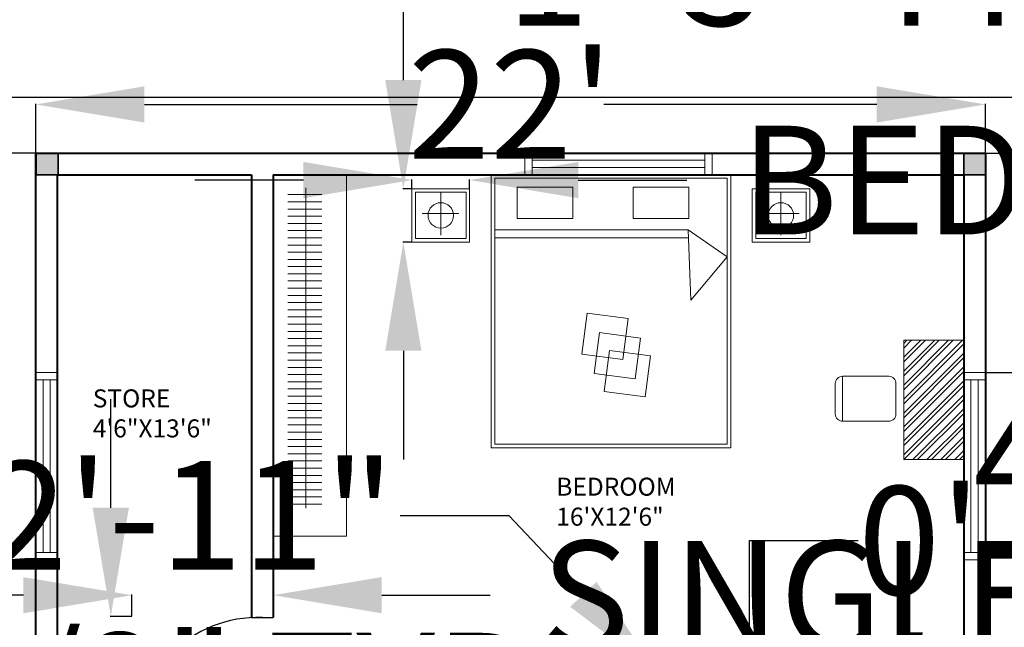
# Model space of a CAD drawing. Units: inches. Extents: x 7323 to 9737, y 2037 to 3322.
# Tile 6 of 19: x 8647 to 8921, y 2540 to 2709. Entities that reach past the tile are written whole.
import ezdxf

# ---------------------------------------------------------------- set-up
doc = ezdxf.new("R2010")
doc.units = ezdxf.units.IN
doc.header["$MEASUREMENT"] = 0
for name, color, linetype, lineweight in [('A-ANNO-DIMS', 2, 'Continuous', 18), ('A-AREA-IDEN', 7, 'Continuous', 18), ('A-COLS', 1, 'Continuous', 35), ('A-DOOR', 4, 'Continuous', 25), ('A-FLOR-CASE', 9, 'Continuous', 20), ('A-FLOR-CASE-PATT', 8, 'Continuous', 13), ('A-FURN', 8, 'Continuous', 18), ('A-FURN-PATT', 252, 'Continuous', 13), ('A-GLAZ', 4, 'Continuous', 18), ('A-WALL', 7, 'Continuous', 40)]:
    doc.layers.add(name, color=color, linetype=linetype, lineweight=lineweight)
doc.layers.add('A-COLS-PATT', color=18, linetype='Continuous', lineweight=13, true_color=0x000000)
doc.styles.get("Standard").update_dxf_attribs({"font": 'arial.ttf'})
doc.dimstyles.get("Standard").update_dxf_attribs({"dimtxt": 30.18, "dimasz": 30.18, "dimexe": 0.18, "dimexo": 0.0625, "dimgap": 0.09, "dimtad": 0, "dimtih": 1, "dimtoh": 1, "dimdec": 0, "dimzin": 0, "dimdsep": 46, "dimlunit": 3, "dimtxsty": 'Standard', "dimcen": 0.09, "dimadec": 0, "dimazin": 0, "dimtfac": 1, "dimtdec": 0, "dimtofl": 0, "dimtmove": 0, "dimatfit": 3, "dimfxl": 1, "dimtolj": 1, "dimtzin": 0, "dimarcsym": 0})

# ---------------------------------------------------------------- blocks, each defined once
blk = doc.blocks.new('*D9')
at = {"layer": 'A-ANNO-DIMS', "color": 0, "lineweight": -2, "transparency": 16777216}
for p, q in [((8651.39, 2671.93), (8651.39, 2685.56)), ((8915.39, 2671.93), (8915.39, 2685.56)), ((8681.57, 2685.38), (8757.44, 2685.38)), ((8885.21, 2685.38), (8809.35, 2685.38))]:
    blk.add_line(p, q, dxfattribs=at)
at = {"layer": 'A-ANNO-DIMS', "color": 0, "transparency": 16777216}
for points in [[(8681.57, 2690.41), (8681.57, 2680.35), (8651.39, 2685.38)], [(8885.21, 2690.41), (8885.21, 2680.35), (8915.39, 2685.38)]]:
    blk.add_solid(points, dxfattribs=at)
at = {"layer": 'Defpoints', "color": 0, "transparency": 16777216}
for p in [(8915.39, 2685.38), (8651.39, 2671.86), (8915.39, 2671.86)]:
    blk.add_point(p, dxfattribs=at)
at = {"layer": 'A-ANNO-DIMS', "color": 0, "transparency": 16777216, "insert": (8783.39, 2685.38), "char_height": 30.18, "attachment_point": 5}
blk.add_mtext("\\A1;22'", dxfattribs=at)
blk = doc.blocks.new('WIN-48')
for p, q in [((0, 0), (0, 6)), ((2, 0), (2, 6)), ((50, 0), (50, 6)), ((52, 0), (52, 6)), ((2, 4), (50, 4)), ((2, 2), (50, 2))]:
    blk.add_line(p, q)
blk = doc.blocks.new('DOOR-36')
for p, q in [((33.01, 39), (39.01, 39)), ((36.01, 5), (0.01, 5)), ((33.01, 3), (0.01, 3)), ((36.01, 5), (36.01, 3)), ((36.01, 3), (39.01, 3)), ((33.01, 0), (39.01, 0))]:
    blk.add_line(p, q)
blk.add_arc((35.01, 4), 35.01, 88.3634, 181.6366)
blk = doc.blocks.new('BED-DOUBLE-REAR')
for p, q in [((1, 60.58), (54.75, 60.58)), ((54.75, 60.58), (65.65, 53.04)), ((55.5, 41.06), (54.75, 60.58)), ((54.83, 58.32), (1, 58.32)), ((65.65, 53.04), (55.5, 41.06))]:
    blk.add_line(p, q)
for points in [[(0, 75.91), (66.65, 75.91), (66.65, 0), (0, 0)], [(1, 74.91), (65.65, 74.91), (65.65, 1), (1, 1)], [(7.24, 72.42), (22.67, 72.42), (22.67, 63.7), (7.24, 63.7)], [(39.52, 72.42), (54.95, 72.42), (54.95, 63.7), (39.52, 63.7)], [(36.59, 24.55), (38.1, 35.92), (26.73, 37.42), (25.22, 26.05)], [(40.02, 19.16), (41.52, 30.53), (30.15, 32.04), (28.64, 20.66)], [(42.82, 14.19), (44.32, 25.56), (32.95, 27.06), (31.44, 15.69)]]:
    blk.add_lwpolyline(points, close=True)
blk = doc.blocks.new('BEDSIDE-TABLE-LARGE')
for p, q in [((8.01, 13.84), (8.01, 1.98)), ((2.84, 7.91), (13.05, 7.91))]:
    blk.add_line(p, q)
for points in [[(0, 14.84), (16.03, 14.84), (16.03, 0), (0, 0)], [(1, 13.84), (15.03, 13.84), (15.03, 1), (1, 1)]]:
    blk.add_lwpolyline(points, close=True)
blk.add_circle((8.01, 7.42), 3.54)
blk = doc.blocks.new('COL-PLAN-6IN')
blk.add_lwpolyline([(0, 6), (0, 6), (6.06, 6), (6.06, 6), (6.06, 0), (6.06, 0), (0, 0), (0, 0)], close=True)
blk = doc.blocks.new('*D39')
at = {"layer": 'A-ANNO-DIMS', "color": 0, "lineweight": -2, "transparency": 16777216}
for p, q in [((8647.94, 2549.03), (8617.76, 2549.03)), ((8678.12, 2543.2), (8678.12, 2549.21)), ((8717.39, 2543.2), (8717.39, 2549.21)), ((8747.57, 2549.03), (8777.75, 2549.03))]:
    blk.add_line(p, q, dxfattribs=at)
at = {"layer": 'A-ANNO-DIMS', "color": 0, "transparency": 16777216}
for points in [[(8647.94, 2554.06), (8647.94, 2544), (8678.12, 2549.03)], [(8747.57, 2554.06), (8747.57, 2544), (8717.39, 2549.03)]]:
    blk.add_solid(points, dxfattribs=at)
at = {"layer": 'Defpoints', "color": 0, "transparency": 16777216}
for p in [(8717.39, 2549.03), (8678.12, 2543.14), (8717.39, 2543.14)]:
    blk.add_point(p, dxfattribs=at)
at = {"layer": 'A-ANNO-DIMS', "color": 0, "transparency": 16777216, "insert": (9057.19, 2549.03), "char_height": 30.18, "attachment_point": 5}
blk.add_mtext('\\A1;SINGLE DOOR 3\'-3 1/2" TYP.', dxfattribs=at)
blk = doc.blocks.new('*D40')
at = {"layer": 'A-ANNO-DIMS', "color": 0, "lineweight": -2, "transparency": 16777216}
for p, q in [((8672.23, 2573.32), (8672.23, 2603.5)), ((8678.06, 2543.14), (8672.05, 2543.14)), ((8678.06, 2503.86), (8672.05, 2503.86)), ((8672.23, 2473.68), (8672.23, 2443.5))]:
    blk.add_line(p, q, dxfattribs=at)
at = {"layer": 'A-ANNO-DIMS', "color": 0, "transparency": 16777216}
for points in [[(8667.2, 2573.32), (8677.26, 2573.32), (8672.23, 2543.14)], [(8667.2, 2473.68), (8677.26, 2473.68), (8672.23, 2503.86)]]:
    blk.add_solid(points, dxfattribs=at)
at = {"layer": 'Defpoints', "color": 0, "transparency": 16777216}
for p in [(8672.23, 2543.14), (8678.12, 2543.14), (8678.12, 2503.86)]:
    blk.add_point(p, dxfattribs=at)
at = {"layer": 'A-ANNO-DIMS', "color": 0, "transparency": 16777216, "insert": (8672.23, 2523.5), "char_height": 30.18, "attachment_point": 5}
blk.add_mtext('\\A1;3\'-3 1/2" TYP.', dxfattribs=at)
blk = doc.blocks.new('*D41')
at = {"layer": 'A-ANNO-DIMS', "color": 0, "lineweight": -2, "transparency": 16777216}
for p, q in [((8661.59, 2428.04), (8661.59, 2458.22)), ((8661.59, 2458.22), (8691.77, 2458.22)), ((8657.46, 2397.86), (8661.77, 2397.86)), ((8657.46, 2369.86), (8661.77, 2369.86)), ((8661.59, 2339.68), (8661.59, 2309.5))]:
    blk.add_line(p, q, dxfattribs=at)
at = {"layer": 'A-ANNO-DIMS', "color": 0, "transparency": 16777216}
for points in [[(8656.56, 2428.04), (8666.62, 2428.04), (8661.59, 2397.86)], [(8656.56, 2339.68), (8666.62, 2339.68), (8661.59, 2369.86)]]:
    blk.add_solid(points, dxfattribs=at)
at = {"layer": 'Defpoints', "color": 0, "transparency": 16777216}
for p in [(8657.39, 2397.86), (8661.59, 2397.86), (8657.39, 2369.86)]:
    blk.add_point(p, dxfattribs=at)
at = {"layer": 'A-ANNO-DIMS', "color": 0, "transparency": 16777216, "insert": (8945.06, 2458.22), "char_height": 30.18, "attachment_point": 5}
blk.add_mtext('\\A1;VENT WINDOW 2\'-4" TYP.', dxfattribs=at)
blk = doc.blocks.new('*D45')
at = {"layer": 'A-ANNO-DIMS', "color": 0, "lineweight": -2, "transparency": 16777216}
for p, q in [((8725.79, 2664.36), (8695.61, 2664.36)), ((8755.97, 2662.02), (8755.97, 2664.54)), ((8772, 2662.02), (8772, 2664.54)), ((8802.18, 2664.36), (8832.36, 2664.36))]:
    blk.add_line(p, q, dxfattribs=at)
at = {"layer": 'A-ANNO-DIMS', "color": 0, "transparency": 16777216}
for points in [[(8725.79, 2669.39), (8725.79, 2659.33), (8755.97, 2664.36)], [(8802.18, 2669.39), (8802.18, 2659.33), (8772, 2664.36)]]:
    blk.add_solid(points, dxfattribs=at)
at = {"layer": 'Defpoints', "color": 0, "transparency": 16777216}
for p in [(8772, 2664.36), (8755.97, 2661.96), (8772, 2661.96)]:
    blk.add_point(p, dxfattribs=at)
at = {"layer": 'A-ANNO-DIMS', "color": 0, "transparency": 16777216, "insert": (9094.8, 2664.36), "char_height": 30.18, "attachment_point": 5}
blk.add_mtext('\\A1;BEDSIDE TABLE 1\'-4" TYP.', dxfattribs=at)
blk = doc.blocks.new('*D46')
at = {"layer": 'A-ANNO-DIMS', "color": 0, "lineweight": -2, "transparency": 16777216}
for p, q in [((8753.57, 2692.14), (8753.57, 2722.32)), ((8753.57, 2722.32), (8783.75, 2722.32)), ((8755.91, 2661.96), (8753.39, 2661.96)), ((8755.91, 2647.12), (8753.39, 2647.12)), ((8753.57, 2616.94), (8753.57, 2586.76))]:
    blk.add_line(p, q, dxfattribs=at)
at = {"layer": 'A-ANNO-DIMS', "color": 0, "transparency": 16777216}
for points in [[(8748.54, 2692.14), (8758.6, 2692.14), (8753.57, 2661.96)], [(8748.54, 2616.94), (8758.6, 2616.94), (8753.57, 2647.12)]]:
    blk.add_solid(points, dxfattribs=at)
at = {"layer": 'Defpoints', "color": 0, "transparency": 16777216}
for p in [(8753.57, 2661.96), (8755.97, 2661.96), (8755.97, 2647.12)]:
    blk.add_point(p, dxfattribs=at)
at = {"layer": 'A-ANNO-DIMS', "color": 0, "transparency": 16777216, "insert": (8874.4, 2722.32), "char_height": 30.18, "attachment_point": 5}
blk.add_mtext('\\A1;1\'-3" TYP.', dxfattribs=at)
blk = doc.blocks.new('*D47')
at = {"layer": 'A-ANNO-DIMS', "color": 0, "lineweight": -2, "transparency": 16777216}
for p, q in [((8809.55, 2464.49), (8779.37, 2464.49)), ((8839.73, 2461.79), (8839.73, 2464.67)), ((8858.14, 2461.79), (8858.14, 2464.67)), ((8888.32, 2464.49), (8918.5, 2464.49))]:
    blk.add_line(p, q, dxfattribs=at)
at = {"layer": 'A-ANNO-DIMS', "color": 0, "transparency": 16777216}
for points in [[(8809.55, 2469.52), (8809.55, 2459.46), (8839.73, 2464.49)], [(8888.32, 2469.52), (8888.32, 2459.46), (8858.14, 2464.49)]]:
    blk.add_solid(points, dxfattribs=at)
at = {"layer": 'Defpoints', "color": 0, "transparency": 16777216}
for p in [(8858.14, 2464.49), (8839.73, 2461.73), (8858.14, 2461.73)]:
    blk.add_point(p, dxfattribs=at)
at = {"layer": 'A-ANNO-DIMS', "color": 0, "transparency": 16777216, "insert": (9164.9, 2464.49), "char_height": 30.18, "attachment_point": 5}
blk.add_mtext('\\A1;ARMCHAIR 1\'-6 1/2" TYP.', dxfattribs=at)
blk = doc.blocks.new('*D48')
at = {"layer": 'A-ANNO-DIMS', "color": 0, "lineweight": -2, "transparency": 16777216}
for p, q in [((8836.96, 2491.91), (8836.96, 2522.09)), ((8836.96, 2522.09), (8867.14, 2522.09)), ((8839.66, 2461.73), (8836.78, 2461.73)), ((8839.66, 2451.75), (8836.78, 2451.75)), ((8836.96, 2421.57), (8836.96, 2391.39))]:
    blk.add_line(p, q, dxfattribs=at)
at = {"layer": 'A-ANNO-DIMS', "color": 0, "transparency": 16777216}
for points in [[(8831.93, 2491.91), (8841.99, 2491.91), (8836.96, 2461.73)], [(8831.93, 2421.57), (8841.99, 2421.57), (8836.96, 2451.75)]]:
    blk.add_solid(points, dxfattribs=at)
at = {"layer": 'Defpoints', "color": 0, "transparency": 16777216}
for p in [(8836.96, 2461.73), (8839.73, 2461.73), (8839.73, 2451.75)]:
    blk.add_point(p, dxfattribs=at)
at = {"layer": 'A-ANNO-DIMS', "color": 0, "transparency": 16777216, "insert": (8970.94, 2522.09), "char_height": 30.18, "attachment_point": 5}
blk.add_mtext('\\A1;0\'-10" TYP.', dxfattribs=at)
blk = doc.blocks.new('*D53')
at = {"layer": 'A-ANNO-DIMS', "color": 0, "lineweight": -2, "transparency": 16777216}
for p, q in [((8826.85, 2511.06), (8796.67, 2511.06)), ((8857.03, 2503.93), (8857.03, 2511.24)), ((8905.03, 2503.93), (8905.03, 2511.24)), ((8935.21, 2511.06), (8965.39, 2511.06))]:
    blk.add_line(p, q, dxfattribs=at)
at = {"layer": 'A-ANNO-DIMS', "color": 0, "transparency": 16777216}
for points in [[(8826.85, 2516.09), (8826.85, 2506.03), (8857.03, 2511.06)], [(8935.21, 2516.09), (8935.21, 2506.03), (8905.03, 2511.06)]]:
    blk.add_solid(points, dxfattribs=at)
at = {"layer": 'Defpoints', "color": 0, "transparency": 16777216}
for p in [(8905.03, 2511.06), (8857.03, 2503.86), (8905.03, 2503.86)]:
    blk.add_point(p, dxfattribs=at)
at = {"layer": 'A-ANNO-DIMS', "color": 0, "transparency": 16777216, "insert": (9261.3, 2511.06), "char_height": 30.18, "attachment_point": 5}
blk.add_mtext('\\A1;INTERIOR WINDOW 4\'-0" TYP.', dxfattribs=at)
blk = doc.blocks.new('*D54')
at = {"layer": 'A-ANNO-DIMS', "color": 0, "lineweight": -2, "transparency": 16777216}
for p, q in [((8849.83, 2534.04), (8849.83, 2564.22)), ((8849.83, 2564.22), (8880.01, 2564.22)), ((8856.96, 2503.86), (8849.65, 2503.86)), ((8856.96, 2497.86), (8849.65, 2497.86)), ((8849.83, 2467.68), (8849.83, 2437.5))]:
    blk.add_line(p, q, dxfattribs=at)
at = {"layer": 'A-ANNO-DIMS', "color": 0, "transparency": 16777216}
for points in [[(8844.8, 2534.04), (8854.86, 2534.04), (8849.83, 2503.86)], [(8844.8, 2467.68), (8854.86, 2467.68), (8849.83, 2497.86)]]:
    blk.add_solid(points, dxfattribs=at)
at = {"layer": 'Defpoints', "color": 0, "transparency": 16777216}
for p in [(8849.83, 2503.86), (8857.03, 2503.86), (8857.03, 2497.86)]:
    blk.add_point(p, dxfattribs=at)
at = {"layer": 'A-ANNO-DIMS', "color": 0, "transparency": 16777216, "insert": (8972.08, 2564.22), "char_height": 30.18, "attachment_point": 5}
blk.add_mtext('\\A1;0\'-6" TYP.', dxfattribs=at)
blk = doc.blocks.new('*D63')
at = {"layer": 'A-ANNO-DIMS', "color": 0, "lineweight": -2, "transparency": 16777216}
for p, q in [((8744.72, 2466.22), (8744.72, 2496.4)), ((8744.72, 2496.4), (8774.9, 2496.4)), ((8741.46, 2436.04), (8744.9, 2436.04)), ((8741.46, 2413.86), (8744.9, 2413.86)), ((8744.72, 2383.68), (8744.72, 2353.5))]:
    blk.add_line(p, q, dxfattribs=at)
at = {"layer": 'A-ANNO-DIMS', "color": 0, "transparency": 16777216}
for points in [[(8739.69, 2466.22), (8749.75, 2466.22), (8744.72, 2436.04)], [(8739.69, 2383.68), (8749.75, 2383.68), (8744.72, 2413.86)]]:
    blk.add_solid(points, dxfattribs=at)
at = {"layer": 'Defpoints', "color": 0, "transparency": 16777216}
for p in [(8741.39, 2436.04), (8744.72, 2436.04), (8741.39, 2413.86)]:
    blk.add_point(p, dxfattribs=at)
at = {"layer": 'A-ANNO-DIMS', "color": 0, "transparency": 16777216, "insert": (9003.76, 2496.4), "char_height": 30.18, "attachment_point": 5}
blk.add_mtext('\\A1;APPLIANCE 1\'-10" TYP.', dxfattribs=at)
blk = doc.blocks.new('*D69')
at = {"layer": 'A-ANNO-DIMS', "color": 0, "lineweight": -2, "transparency": 16777216}
for p, q in [((8836.58, 2472.89), (8836.58, 2503.07)), ((8836.58, 2503.07), (8866.76, 2503.07)), ((8839.88, 2442.71), (8836.4, 2442.71)), ((8839.88, 2420.33), (8836.4, 2420.33)), ((8836.58, 2390.15), (8836.58, 2359.97))]:
    blk.add_line(p, q, dxfattribs=at)
at = {"layer": 'A-ANNO-DIMS', "color": 0, "transparency": 16777216}
for points in [[(8831.55, 2472.89), (8841.61, 2472.89), (8836.58, 2442.71)], [(8831.55, 2390.15), (8841.61, 2390.15), (8836.58, 2420.33)]]:
    blk.add_solid(points, dxfattribs=at)
at = {"layer": 'Defpoints', "color": 0, "transparency": 16777216}
for p in [(8836.58, 2442.71), (8839.94, 2442.71), (8839.94, 2420.33)]:
    blk.add_point(p, dxfattribs=at)
at = {"layer": 'A-ANNO-DIMS', "color": 0, "transparency": 16777216, "insert": (9169.54, 2503.07), "char_height": 30.18, "attachment_point": 5}
blk.add_mtext('\\A1;COFFEE TABLE 1\'-10 1/2" TYP.', dxfattribs=at)
blk = doc.blocks.new('*D81')
at = {"layer": 'A-ANNO-DIMS', "color": 0, "lineweight": -2, "transparency": 16777216}
for p, q in [((8651.33, 2671.86), (8587.16, 2671.86)), ((8587.34, 2641.68), (8587.34, 2443.36)), ((8587.34, 2214.04), (8587.34, 2412.36)), ((8651.33, 2183.86), (8587.16, 2183.86))]:
    blk.add_line(p, q, dxfattribs=at)
at = {"layer": 'A-ANNO-DIMS', "color": 0, "transparency": 16777216}
for points in [[(8582.31, 2641.68), (8592.37, 2641.68), (8587.34, 2671.86)], [(8582.31, 2214.04), (8592.37, 2214.04), (8587.34, 2183.86)]]:
    blk.add_solid(points, dxfattribs=at)
at = {"layer": 'Defpoints', "color": 0, "transparency": 16777216}
for p in [(8587.34, 2671.86), (8651.39, 2671.86), (8651.39, 2183.86)]:
    blk.add_point(p, dxfattribs=at)
at = {"layer": 'A-ANNO-DIMS', "color": 0, "transparency": 16777216, "insert": (8587.34, 2427.86), "char_height": 30.18, "attachment_point": 5}
blk.add_mtext('\\A1;40\'-8"', dxfattribs=at)
blk = doc.blocks.new('*D100')
at = {"layer": 'A-ANNO-DIMS', "color": 0, "lineweight": -2, "transparency": 16777216}
for p, q in [((9007.88, 2687.3), (8587.16, 2687.3)), ((8587.34, 2657.12), (8587.34, 2615.8)), ((8587.34, 2543.49), (8587.34, 2584.8)), ((9008.12, 2513.31), (8587.16, 2513.31))]:
    blk.add_line(p, q, dxfattribs=at)
at = {"layer": 'A-ANNO-DIMS', "color": 0, "transparency": 16777216}
for points in [[(8582.31, 2657.12), (8592.37, 2657.12), (8587.34, 2687.3)], [(8582.31, 2543.49), (8592.37, 2543.49), (8587.34, 2513.31)]]:
    blk.add_solid(points, dxfattribs=at)
at = {"layer": 'Defpoints', "color": 0, "transparency": 16777216}
for p in [(9007.95, 2687.3), (8587.34, 2513.31), (9008.18, 2513.31)]:
    blk.add_point(p, dxfattribs=at)
at = {"layer": 'A-ANNO-DIMS', "color": 0, "transparency": 16777216, "insert": (8587.34, 2600.3), "char_height": 30.18, "attachment_point": 5}
blk.add_mtext('\\A1;14\'-6"', dxfattribs=at)
blk = doc.blocks.new('*D114')
at = {"layer": 'A-ANNO-DIMS', "color": 0, "lineweight": -2, "transparency": 16777216}
for p, q in [((8915.46, 2671.86), (9307.45, 2671.86)), ((9307.27, 2641.68), (9307.27, 2641.04)), ((8915.46, 2610.86), (9307.45, 2610.86)), ((9307.27, 2610.86), (9307.27, 2580.68)), ((9307.27, 2580.68), (9277.09, 2580.68))]:
    blk.add_line(p, q, dxfattribs=at)
at = {"layer": 'A-ANNO-DIMS', "color": 0, "transparency": 16777216}
for points in [[(9302.24, 2641.68), (9312.3, 2641.68), (9307.27, 2671.86)], [(9302.24, 2641.04), (9312.3, 2641.04), (9307.27, 2610.86)]]:
    blk.add_solid(points, dxfattribs=at)
at = {"layer": 'Defpoints', "color": 0, "transparency": 16777216}
for p in [(8915.39, 2671.86), (8915.39, 2610.86), (9307.27, 2610.86)]:
    blk.add_point(p, dxfattribs=at)
at = {"layer": 'A-ANNO-DIMS', "color": 0, "transparency": 16777216, "insert": (9236.89, 2580.68), "char_height": 30.18, "attachment_point": 5}
blk.add_mtext('\\A1;5\'-1"', dxfattribs=at)
blk = doc.blocks.new('*D124')
at = {"layer": 'A-ANNO-DIMS', "color": 0, "lineweight": -2, "transparency": 16777216}
for p, q in [((8752.73, 2571.2), (8782.91, 2571.2)), ((8782.91, 2571.2), (8803.63, 2549.26)), ((8848.3, 2501.86), (8848.48, 2501.86)), ((8848.39, 2501.77), (8848.39, 2501.95))]:
    blk.add_line(p, q, dxfattribs=at)
at = {"layer": 'A-ANNO-DIMS', "color": 0, "transparency": 16777216}
blk.add_solid([(8807.29, 2552.71), (8799.97, 2545.81), (8824.35, 2527.32)], dxfattribs=at)
at = {"layer": 'Defpoints', "color": 0, "transparency": 16777216}
for p in [(8824.35, 2527.32), (8848.39, 2501.86)]:
    blk.add_point(p, dxfattribs=at)
at = {"layer": 'A-ANNO-DIMS', "color": 0, "transparency": 16777216, "insert": (8653.33, 2571.2), "char_height": 30.18, "attachment_point": 5}
blk.add_mtext('\\A1;4X R2\'-11"', dxfattribs=at)
blk = doc.blocks.new('*D126')
at = {"layer": 'A-ANNO-DIMS', "color": 0, "lineweight": -2, "transparency": 16777216}
for p, q in [((9109.28, 2586.63), (9139.46, 2586.63)), ((9139.46, 2586.63), (9160.18, 2564.69)), ((9204.86, 2517.3), (9205.04, 2517.3)), ((9204.95, 2517.21), (9204.95, 2517.39))]:
    blk.add_line(p, q, dxfattribs=at)
at = {"layer": 'A-ANNO-DIMS', "color": 0, "transparency": 16777216}
blk.add_solid([(9163.84, 2568.15), (9156.52, 2561.24), (9180.9, 2542.75)], dxfattribs=at)
at = {"layer": 'Defpoints', "color": 0, "transparency": 16777216}
for p in [(9180.9, 2542.75), (9204.95, 2517.3)]:
    blk.add_point(p, dxfattribs=at)
at = {"layer": 'A-ANNO-DIMS', "color": 0, "transparency": 16777216, "insert": (9009.88, 2586.63), "char_height": 30.18, "attachment_point": 5}
blk.add_mtext('\\A1;4X R2\'-11"', dxfattribs=at)

msp = doc.modelspace()

# ---------------------------------------------------------------- hatches: boundary and pattern name
at = {"layer": 'A-COLS-PATT'}
h = msp.add_hatch(color=256, dxfattribs=at)
h.dxf.hatch_style = 1
h.paths.add_polyline_path([(8915.39, 2189.86), (8908.77, 2189.86), (8908.77, 2183.86), (8915.39, 2183.86)])
h.paths.add_polyline_path([(8657.61, 2189.86), (8651.55, 2189.86), (8651.55, 2183.86), (8657.61, 2183.86)])
h.paths.add_polyline_path([(8814.13, 2189.86), (8807.39, 2189.86), (8807.39, 2183.86), (8814.13, 2183.86)])
h.paths.add_polyline_path([(8813.39, 2317.86), (8807.36, 2317.86), (8807.36, 2311.86), (8813.39, 2311.86)])
h.paths.add_polyline_path([(8915.34, 2313.13), (8909.39, 2313.13), (8909.39, 2307.13), (8915.34, 2307.13)])
h.paths.add_polyline_path([(8657.62, 2317.86), (8657.39, 2317.86), (8657.39, 2318.08), (8651.55, 2318.08), (8651.55, 2312.08), (8657.62, 2312.08)])
h.paths.add_polyline_path([(8915.39, 2671.84), (8909.37, 2671.84), (8909.37, 2665.86), (8909.39, 2665.86), (8915.39, 2665.84)])
h.paths.add_polyline_path([(8657.59, 2671.81), (8651.52, 2671.81), (8651.52, 2665.81), (8657.39, 2665.81), (8657.39, 2665.86)])
h.paths.add_polyline_path([(8915.28, 2503.94), (8909.39, 2503.94), (8909.39, 2503.86), (8909.22, 2497.94), (8915.28, 2497.94)])
h.paths.add_polyline_path([(8657.53, 2503.86), (8657.39, 2503.86), (8651.46, 2503.96), (8651.46, 2497.96), (8657.53, 2497.96)])
h.paths.add_polyline_path([(9014.24, 2519.3), (9013.95, 2519.3), (9008.18, 2519.31), (9008.18, 2513.31), (9014.24, 2513.31)])
h.paths.add_polyline_path([(9013.95, 2687.3), (9007.95, 2687.3), (9007.95, 2681.3), (9013.95, 2681.3)])
h.paths.add_polyline_path([(9271.95, 2687.3), (9266.01, 2687.3), (9266.01, 2681.35), (9271.95, 2681.35)])
h.paths.add_polyline_path([(9271.95, 2205.3), (9265.32, 2205.3), (9265.32, 2199.3), (9271.95, 2199.3)])
h.paths.add_polyline_path([(9170.68, 2205.3), (9163.95, 2205.3), (9163.95, 2199.3), (9170.68, 2199.3)])
h.paths.add_polyline_path([(9013.95, 2205.3), (9007.95, 2205.3), (9007.95, 2199.3), (9013.95, 2199.3)])
h.paths.add_polyline_path([(9271.95, 2519.51), (9265.95, 2519.51), (9265.95, 2519.3), (9265.93, 2513.51), (9271.95, 2513.51)])
h.paths.add_polyline_path([(9271.95, 2328.64), (9265.95, 2328.64), (9265.95, 2322.64), (9271.95, 2322.64)])
h.paths.add_polyline_path([(9014.35, 2333.3), (9013.95, 2333.3), (9013.95, 2333.58), (9008.29, 2333.58), (9008.29, 2327.58), (9014.35, 2327.58)])
at = {"layer": 'A-FLOR-CASE-PATT'}
h = msp.add_hatch(dxfattribs=at)
h.set_pattern_fill('ANSI31', color=256, scale=16.001946, angle=-45, style=0)
h.paths.add_polyline_path([(8721.41, 2574.29), (8730.91, 2574.29), (8730.91, 2660.35), (8721.41, 2660.35)])
at = {"layer": 'A-FURN-PATT'}
h = msp.add_hatch(dxfattribs=at)
h.set_pattern_fill('ANSI32', color=256, scale=7.3)
h.set_pattern_definition([(45, (1460.701, -469.2936), (-1.9357048, 1.9357048), []), (45, (1461.9915, -469.2936), (-1.9357048, 1.9357048), [])])
h.paths.add_polyline_path([(8892.71, 2586.7), (8909.39, 2586.7), (8909.39, 2619.84), (8892.71, 2619.84)])

# ---------------------------------------------------------------- linework, layer by layer
at = {"layer": 'A-FLOR-CASE'}
msp.add_line((8726.42, 2662.23), (8726.42, 2573.2), dxfattribs=at)
msp.add_lwpolyline([(8717.39, 2665.86), (8737.81, 2665.86), (8737.81, 2565.39), (8717.39, 2565.39)], close=True, dxfattribs=at)
at = {"layer": 'A-FURN'}
msp.add_line((8875.66, 2609.85), (8875.66, 2597.37), dxfattribs=at)
msp.add_lwpolyline([(8909.39, 2619.84), (8892.71, 2619.84), (8892.71, 2586.7), (8909.39, 2586.7)], close=True, dxfattribs=at)
msp.add_lwpolyline([(8873.66, 2607.85, -0.414214), (8875.66, 2609.85), (8888.54, 2609.85, -0.414214), (8890.54, 2607.85), (8890.54, 2599.37, -0.414214), (8888.54, 2597.37), (8875.66, 2597.37, -0.414214), (8873.66, 2599.37)], format="xyb", close=True, dxfattribs=at)
at = {"layer": 'A-WALL'}
for p, q in [((8651.39, 2183.86), (8651.39, 2671.86)), ((8651.39, 2671.86), (8915.39, 2671.86)), ((8915.39, 2671.86), (8915.39, 2183.86)), ((8657.39, 2665.86), (8711.39, 2665.86)), ((8657.39, 2503.86), (8657.39, 2665.86)), ((8711.39, 2665.86), (8711.39, 2542.82)), ((8717.39, 2665.86), (8717.39, 2542.86)), ((8717.39, 2665.86), (8909.39, 2665.86)), ((8909.39, 2665.86), (8909.39, 2503.86))]:
    msp.add_line(p, q, dxfattribs=at)

# ---------------------------------------------------------------- block references
at = {"layer": 'A-COLS'}
for p in [(8909.37, 2665.84), (8651.52, 2665.81)]:
    msp.add_blockref('COL-PLAN-6IN', p, dxfattribs=at)
at = {"layer": 'A-DOOR'}
msp.add_blockref('DOOR-36', (8678.38, 2503.86), dxfattribs=at)
at = {"layer": 'A-FURN'}
for name, p in [('BED-DOUBLE-REAR', (8777.98, 2589.95)), ('BEDSIDE-TABLE-LARGE', (8755.97, 2647.12)), ('BEDSIDE-TABLE-LARGE', (8850.53, 2647.12))]:
    msp.add_blockref(name, p, dxfattribs=at)
at = {"layer": 'A-GLAZ'}
msp.add_blockref('WIN-48', (8787.39, 2665.86), dxfattribs=at)
for p, rotation in [((8657.39, 2558.86), 89.99999999999191), ((8909.39, 2610.86), 270.0000000000078)]:
    msp.add_blockref('WIN-48', p, dxfattribs=dict(at, rotation=rotation))

# ---------------------------------------------------------------- texts
at = {"layer": 'A-AREA-IDEN', "char_height": 5, "attachment_point": 1}
for s, insert in [('STORE\\P4\'6"X13\'6"', (8667.22, 2606.21)), ('BEDROOM\\P16\'X12\'6"', (8796.09, 2581.68))]:
    msp.add_mtext_dynamic_manual_height_columns(s, width=44.1759, gutter_width=1, heights=[0], dxfattribs=dict(at, insert=insert))

# ---------------------------------------------------------------- dimensions: what is measured, and where the dimension line sits
at = {"layer": 'A-ANNO-DIMS'}
for base, p1, p2, text, picture, middle in [((8753.57, 2661.96), (8755.97, 2647.12), (8755.97, 2661.96), '<> TYP.', '*D46', (8874.4, 2722.32)), ((8836.58, 2442.71), (8839.94, 2420.33), (8839.94, 2442.71), 'COFFEE TABLE <> TYP.', '*D69', (9169.54, 2503.07)), ((8849.83, 2503.86), (8857.03, 2497.86), (8857.03, 2503.86), '<> TYP.', '*D54', (8972.08, 2564.22)), ((8672.23, 2543.14), (8678.12, 2503.86), (8678.12, 2543.14), '<> TYP.', '*D40', (8672.23, 2523.5)), ((8744.72, 2436.04), (8741.39, 2413.86), (8741.39, 2436.04), 'APPLIANCE <> TYP.', '*D63', (9003.76, 2496.4)), ((8836.96, 2461.73), (8839.73, 2451.75), (8839.73, 2461.73), '<> TYP.', '*D48', (8970.94, 2522.09)), ((8661.59, 2397.86), (8657.39, 2369.86), (8657.39, 2397.86), 'VENT WINDOW <> TYP.', '*D41', (8945.06, 2458.22))]:
    dim = msp.add_linear_dim(base=base, p1=p1, p2=p2, angle=90, text=text, dimstyle='Standard', override={"dimdec": 1, "dimlfac": 1, "dimrnd": 0, "dimzin": 1, "dimdsep": 46, "dimlunit": 4, "dimfrac": 2}, dxfattribs=at)
    dim.commit()
    dim.dimension.update_dxf_attribs({"geometry": picture, "text_midpoint": middle})
for base, p1, p2, text, picture, middle in [((8772, 2664.36), (8755.97, 2661.96), (8772, 2661.96), 'BEDSIDE TABLE <> TYP.', '*D45', (9094.8, 2664.36)), ((8717.39, 2549.03), (8678.12, 2543.14), (8717.39, 2543.14), 'SINGLE DOOR <> TYP.', '*D39', (9057.19, 2549.03)), ((8905.03, 2511.06), (8857.03, 2503.86), (8905.03, 2503.86), 'INTERIOR WINDOW <> TYP.', '*D53', (9261.3, 2511.06)), ((8858.14, 2464.49), (8839.73, 2461.73), (8858.14, 2461.73), 'ARMCHAIR <> TYP.', '*D47', (9164.9, 2464.49))]:
    dim = msp.add_linear_dim(base=base, p1=p1, p2=p2, text=text, dimstyle='Standard', override={"dimdec": 1, "dimlfac": 1, "dimrnd": 0, "dimzin": 1, "dimdsep": 46, "dimlunit": 4, "dimfrac": 2}, dxfattribs=at)
    dim.commit()
    dim.dimension.update_dxf_attribs({"geometry": picture, "text_midpoint": middle})
dim = msp.add_linear_dim(base=(8915.39, 2685.38), p1=(8651.39, 2671.86), p2=(8915.39, 2671.86), dimstyle='Standard', override={"dimclrd": 0, "dimclre": 0, "dimclrt": 0}, dxfattribs=at)
dim.commit()
dim.dimension.update_dxf_attribs({"geometry": '*D9', "text_midpoint": (8783.39, 2685.38)})
for base, p1, p2, picture, middle in [((8587.34, 2513.31), (9007.95, 2687.3), (9008.18, 2513.31), '*D100', (8587.34, 2600.3)), ((8587.34, 2671.86), (8651.39, 2183.86), (8651.39, 2671.86), '*D81', (8587.34, 2427.86)), ((9307.27, 2610.86), (8915.39, 2671.86), (8915.39, 2610.86), '*D114', (9236.89, 2580.68))]:
    dim = msp.add_linear_dim(base=base, p1=p1, p2=p2, angle=90, dimstyle='Standard', override={"dimdec": 1, "dimlfac": 1, "dimrnd": 0, "dimzin": 1, "dimdsep": 46, "dimlunit": 4, "dimfrac": 2}, dxfattribs=at)
    dim.commit()
    dim.dimension.update_dxf_attribs({"geometry": picture, "text_midpoint": middle})
for center, mpoint, picture, middle in [((9204.95, 2517.3), (9180.9, 2542.75), '*D126', (9009.88, 2586.63)), ((8848.39, 2501.86), (8824.35, 2527.32), '*D124', (8653.33, 2571.2))]:
    dim = msp.add_radius_dim(center=center, mpoint=mpoint, text='4X <>', dimstyle='Standard', override={"dimdec": 1, "dimlfac": 1, "dimrnd": 0, "dimzin": 1, "dimdsep": 46, "dimlunit": 4, "dimfrac": 2}, dxfattribs=at)
    dim.commit()
    dim.dimension.update_dxf_attribs({"geometry": picture, "text_midpoint": middle})

doc.saveas('drawing.dxf')
